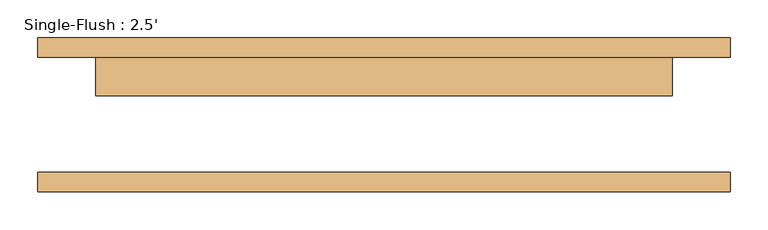
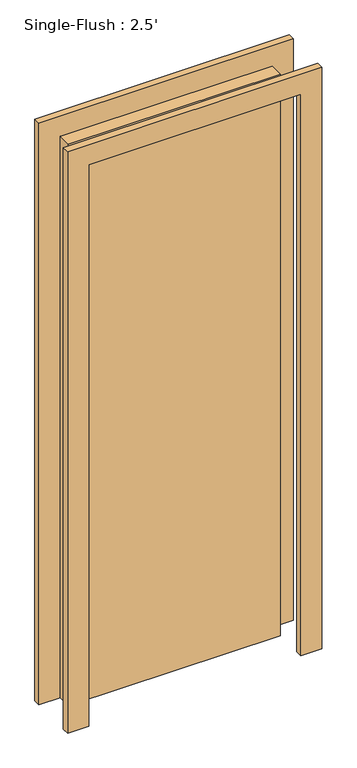
"""IFC4 building model written with IfcOpenShell, lengths in millimetres: door geometry, Single-Flush : 2.5'."""

from ifc_helpers import new_model, si_unit, frame, origin, origin_with_axes, place, context, project, spatial, polyline, outline, extrude, source, transform, mapped, element, save


def single_flush_2_5_a9addea7(model_context):
    return source(origin(), model_context, "Body", "SweptSolid", [
        extrude(outline(polyline([(2209.8, -457.2), (0.0, -457.2), (0.0, -381.0), (2133.6, -381.0), (2133.6, 381.0), (0.0, 381.0), (0.0, 457.2), (2209.8, 457.2), (2209.8, -457.2)])), frame((0.0, 76.2, 0.0), z_axis=(0.0, 1.0, 0.0), x_axis=(0.0, 0.0, 1.0)), (0.0, 0.0, 1.0), 25.4),
        extrude(outline(polyline([(2209.8, 457.2), (2209.8, -457.2), (0.0, -457.2), (0.0, -381.0), (2133.6, -381.0), (2133.6, 381.0), (0.0, 381.0), (0.0, 457.2), (2209.8, 457.2)])), frame((0.0, -101.6, 0.0), z_axis=(0.0, 1.0, 0.0), x_axis=(0.0, 0.0, 1.0)), (0.0, 0.0, 1.0), 25.4),
        extrude(outline(polyline([(381.0, 25.4), (-381.0, 25.4), (-381.0, 76.2), (381.0, 76.2), (381.0, 25.4)])), origin_with_axes(), (0.0, 0.0, 1.0), 2133.6),
    ])


if __name__ == "__main__":
    model = new_model("IFC4")
    model_context = context("Model", 3, world=origin())
    ifc_project = project(units=[si_unit("LENGTHUNIT", "METRE", prefix="MILLI")], contexts=[model_context])
    site = spatial("IfcSite", under=ifc_project)
    building = spatial("IfcBuilding", under=site)
    placement = place(None, origin())
    single_flush_2_5_shape = single_flush_2_5_a9addea7(model_context)
    element("IfcDoor", 1, ObjectType="Single-Flush : 2.5'", at=placement, inside=building, context=model_context, shape_type="MappedRepresentation", body=[
        mapped(single_flush_2_5_shape, transform((0.0, 0.0, 0.0), x_axis=(1.0, 0.0, 0.0), y_axis=(0.0, 1.0, 0.0), z_axis=(0.0, 0.0, 1.0))),
    ])
    save(model, "model.ifc")

# Revit data of these elements
# Type "Single-Flush : 2.5'"
#   Type Mark = "8"
#   Construction Type Id = "MDOOR"
#   Assembly Code = "C1020"
#   Analytic Construction = "Metal"
#   Thickness = 0' - 2"
#   Heat Transfer Coefficient (U) = 0.651978 BTU/(h·ft²·°F)
#   Height = 7' - 0"
#   Trim Projection Ext = 0' - 1"
#   Trim Projection Int = 0' - 1"
#   Trim Width = 0' - 3"
#   Width = 2' - 6"
#   Define Thermal Properties by = 1
#   Door Material = Door - Panel
#   Frame Material = Door - Frame
#   Visual Light Transmittance = 0
#   Solar Heat Gain Coefficient = 0
#   Function = (empty or 0)
#   Wall Closure = (empty or 0)
# Element 1 (IfcDoor, "Single-Flush : 2.5'")
#   Materials on its faces: "Door - Frame", "Door - Panel"
# Materials
#   "Door - Panel": class "Wood", colour RGB 210 159 95, transparency 0
#   "Door - Frame": colour RGB 118 70 51, transparency 0
